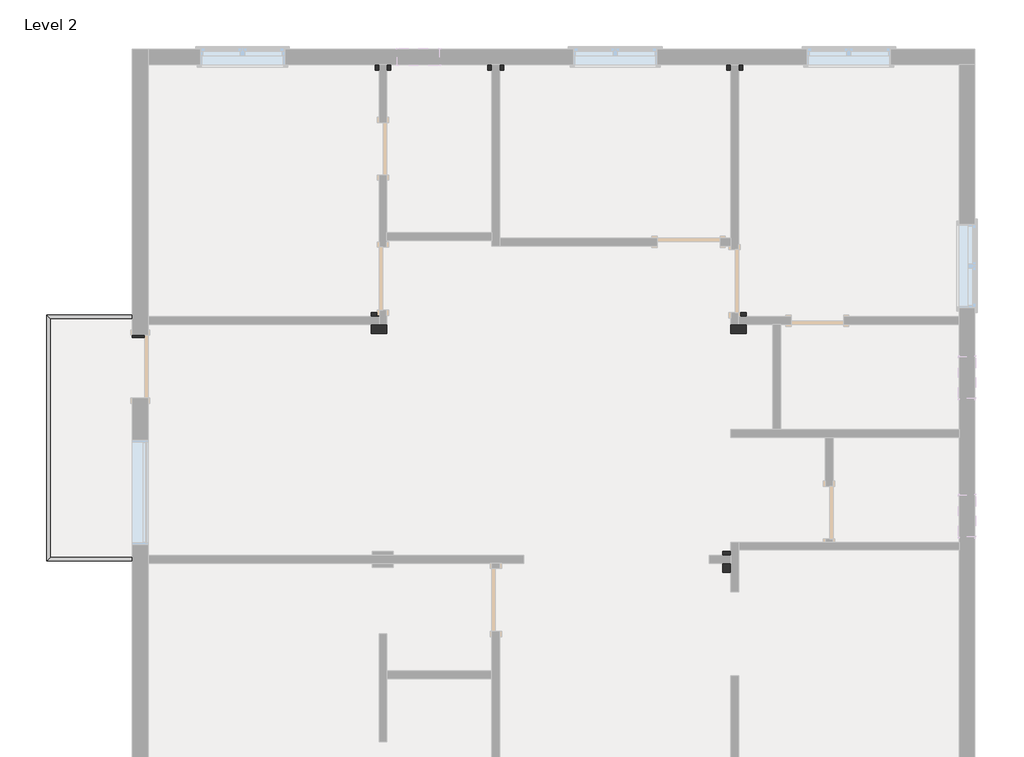
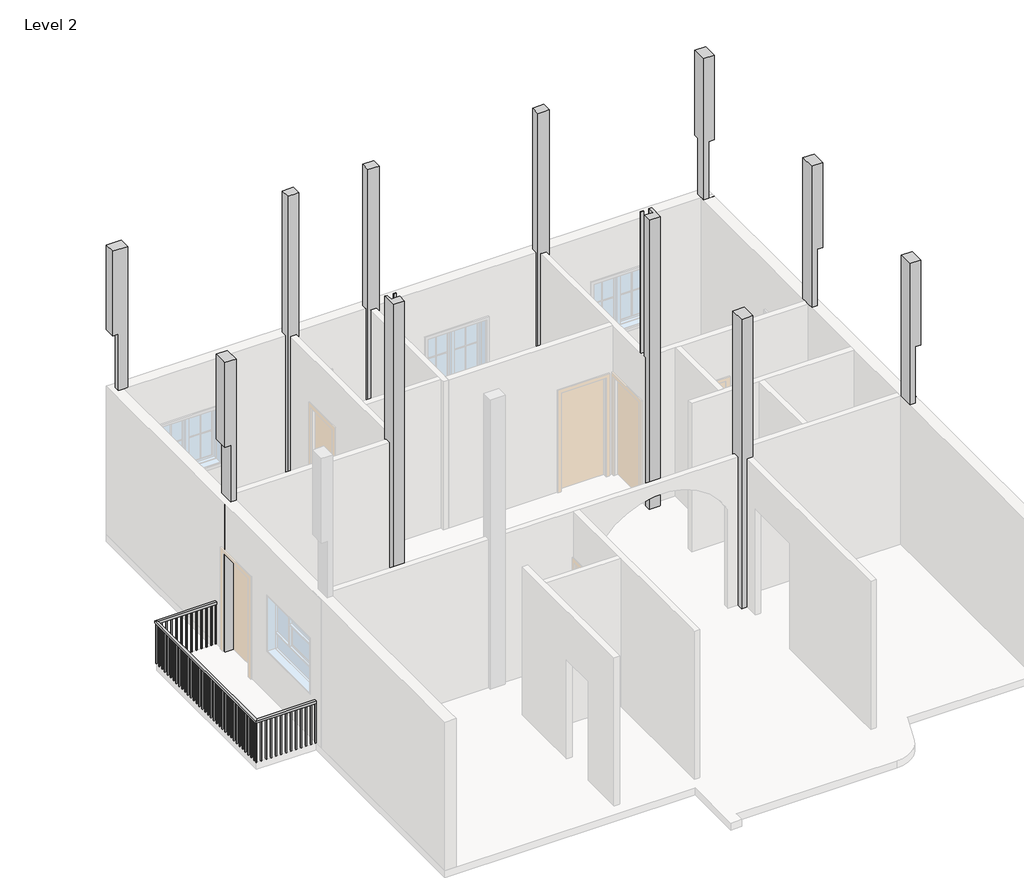
# One storey, part 3 of 4: 11 columns, 1 railing.
"""IFC4 building model written with IfcOpenShell, lengths in millimetres."""

from ifc_helpers import new_model, si_unit, frame, origin, place, context, project, spatial, polyline, outline, extrude, faceted_brep, element, save

model = new_model("IFC4")

# Units and contexts
model_context = context("Model", 3, world=origin())
ifc_project = project(units=[si_unit("LENGTHUNIT", "METRE", prefix="MILLI")], contexts=[model_context])

# Site, building, storey
site = spatial("IfcSite", under=ifc_project)
building = spatial("IfcBuilding", under=site)
storey = spatial("IfcBuildingStorey", under=building, Name="Level 2", Elevation=3200.4)

# Columns
placement = place(None, origin())
element("IfcColumn", 1, ObjectType="Rectangular Column : 9\" x 12\"", at=placement, inside=storey, context=model_context, shape_type="Brep", body=[
    faceted_brep([(-14591.1678125, 13531.616018, 3200.4), (-14591.1678125, 13303.016018, 3200.4), (-14667.3678125, 13303.016018, 3200.4), (-14667.3678125, 13531.616018, 3200.4), (-14591.1678125, 13531.616018, 6400.8), (-14591.1678125, 13417.316018, 6400.8), (-14591.1678125, 13417.316018, 7620.0), (-14591.1678125, 13531.616018, 7620.0), (-14591.1678125, 13531.616018, 9448.8), (-14591.1678125, 13303.016018, 9448.8), (-14895.9678125, 13303.016018, 9448.8), (-14895.9678125, 13303.016018, 7620.0), (-14781.6678125, 13303.016018, 7620.0), (-14781.6678125, 13303.016018, 6400.8), (-14667.3678125, 13303.016018, 6400.8), (-14895.9678125, 13531.616018, 9448.8), (-14895.9678125, 13531.616018, 7620.0), (-14895.9678125, 13417.316018, 7620.0), (-14667.3678125, 13417.316018, 6400.8), (-14667.3678125, 13531.616018, 6400.8), (-14781.6678125, 13417.316018, 6400.8), (-14781.6678125, 13417.316018, 7620.0)], [[[0, 1, 2, 3]], [[1, 0, 4, 5, 6, 7, 8, 9]], [[1, 9, 10, 11, 12, 13, 14, 2]], [[10, 15, 16, 17, 11]], [[15, 8, 7, 16]], [[9, 8, 15, 10]], [[3, 2, 14, 18, 19]], [[14, 13, 20, 18]], [[12, 21, 20, 13]], [[21, 12, 11, 17]], [[5, 18, 20, 21, 6]], [[18, 5, 4, 19]], [[6, 21, 17, 16, 7]], [[0, 3, 19, 4]]]),
])
element("IfcColumn", 2, ObjectType="Rectangular Column : 9\" x 12\"", at=placement, inside=storey, context=model_context, shape_type="Brep", body=[
    faceted_brep([(-11371.7178125, 13226.816018, 3200.4), (-11371.7178125, 13303.016018, 3200.4), (-11314.5678125, 13303.016018, 3200.4), (-11314.5678125, 13226.816018, 3200.4), (-11143.1178125, 13226.816018, 9448.8), (-11143.1178125, 13226.816018, 3200.4), (-11143.1178125, 13303.016018, 3200.4), (-11143.1178125, 13303.016018, 6400.8), (-11143.1178125, 13417.316018, 6400.8), (-11143.1178125, 13417.316018, 9448.8), (-11257.4178125, 13226.816018, 9448.8), (-11371.7178125, 13226.816018, 9448.8), (-11371.7178125, 13226.816018, 6400.8), (-11314.5678125, 13226.816018, 6400.8), (-11257.4178125, 13226.816018, 6400.8), (-11200.2678125, 13226.816018, 6400.8), (-11200.2678125, 13226.816018, 3200.4), (-11371.7178125, 13417.316018, 9448.8), (-11371.7178125, 13417.316018, 6400.8), (-11371.7178125, 13303.016018, 6400.8), (-11314.5678125, 13303.016018, 6400.8), (-11200.2678125, 13303.016018, 6400.8), (-11200.2678125, 13303.016018, 3200.4)], [[[0, 1, 2, 3]], [[4, 5, 6, 7, 8, 9]], [[5, 4, 10, 11, 12, 0, 3, 13, 14, 15, 16]], [[0, 12, 11, 17, 18, 19, 1]], [[11, 10, 4, 9, 17]], [[1, 19, 20, 2]], [[20, 19, 18, 8, 7, 21]], [[20, 13, 3, 2]], [[15, 21, 22, 16]], [[13, 20, 21, 15, 14]], [[6, 5, 16, 22]], [[7, 6, 22, 21]], [[9, 8, 18, 17]]]),
])
element("IfcColumn", 3, ObjectType="Rectangular Column : 9\" x 12\"", at=placement, inside=storey, context=model_context, shape_type="Brep", body=[
    faceted_brep([(-9733.4178125, 13226.816018, 3200.4), (-9733.4178125, 13303.016018, 3200.4), (-9676.2678125, 13303.016018, 3200.4), (-9676.2678125, 13226.816018, 3200.4), (-9504.8178125, 13226.816018, 9448.8), (-9504.8178125, 13226.816018, 3200.4), (-9504.8178125, 13303.016018, 3200.4), (-9504.8178125, 13303.016018, 6400.8), (-9504.8178125, 13417.316018, 6400.8), (-9504.8178125, 13417.316018, 9448.8), (-9733.4178125, 13226.816018, 9448.8), (-9676.2678125, 13226.816018, 6400.8), (-9561.9678125, 13226.816018, 6400.8), (-9561.9678125, 13226.816018, 3200.4), (-9733.4178125, 13417.316018, 9448.8), (-9733.4178125, 13417.316018, 6400.8), (-9733.4178125, 13303.016018, 6400.8), (-9676.2678125, 13303.016018, 6400.8), (-9561.9678125, 13303.016018, 6400.8), (-9561.9678125, 13303.016018, 3200.4)], [[[0, 1, 2, 3]], [[4, 5, 6, 7, 8, 9]], [[5, 4, 10, 0, 3, 11, 12, 13]], [[0, 10, 14, 15, 16, 1]], [[10, 4, 9, 14]], [[1, 16, 17, 2]], [[17, 16, 15, 8, 7, 18]], [[17, 11, 3, 2]], [[12, 18, 19, 13]], [[11, 17, 18, 12]], [[6, 5, 13, 19]], [[7, 6, 19, 18]], [[9, 8, 15, 14]]]),
])
element("IfcColumn", 4, ObjectType="Rectangular Column : 9\" x 12\"", at=placement, inside=storey, context=model_context, shape_type="Brep", body=[
    faceted_brep([(-6266.3178125, 13226.816018, 3200.4), (-6266.3178125, 13303.016018, 3200.4), (-6209.1678125, 13303.016018, 3200.4), (-6209.1678125, 13226.816018, 3200.4), (-6037.7178125, 13226.816018, 9448.8), (-6037.7178125, 13226.816018, 6400.8), (-6037.7178125, 13226.816018, 3200.4), (-6037.7178125, 13303.016018, 3200.4), (-6037.7178125, 13303.016018, 6400.8), (-6037.7178125, 13417.316018, 6400.8), (-6037.7178125, 13417.316018, 9448.8), (-6152.0178125, 13226.816018, 9448.8), (-6266.3178125, 13226.816018, 9448.8), (-6209.1678125, 13226.816018, 6400.8), (-6152.0178125, 13226.816018, 6400.8), (-6094.8678125, 13226.816018, 6400.8), (-6094.8678125, 13226.816018, 3200.4), (-6266.3178125, 13417.316018, 9448.8), (-6266.3178125, 13417.316018, 6400.8), (-6266.3178125, 13303.016018, 6400.8), (-6209.1678125, 13303.016018, 6400.8), (-6094.8678125, 13303.016018, 6400.8), (-6094.8678125, 13303.016018, 3200.4)], [[[0, 1, 2, 3]], [[4, 5, 6, 7, 8, 9, 10]], [[6, 5, 4, 11, 12, 0, 3, 13, 14, 15, 16]], [[0, 12, 17, 18, 19, 1]], [[12, 11, 4, 10, 17]], [[1, 19, 20, 2]], [[20, 19, 18, 9, 8, 21]], [[20, 13, 3, 2]], [[15, 21, 22, 16]], [[13, 20, 21, 15, 14]], [[7, 6, 16, 22]], [[8, 7, 22, 21]], [[10, 9, 18, 17]]]),
])
element("IfcColumn", 5, ObjectType="Rectangular Column : 9\" x 12\"", at=placement, inside=storey, context=model_context, shape_type="Brep", body=[
    faceted_brep([(-2665.8678125, 13226.816018, 3200.4), (-2894.4678125, 13226.816018, 3200.4), (-2894.4678125, 13303.016018, 3200.4), (-2665.8678125, 13303.016018, 3200.4), (-2894.4678125, 13531.616018, 9448.8), (-2665.8678125, 13531.616018, 9448.8), (-2665.8678125, 13531.616018, 7620.0), (-2894.4678125, 13531.616018, 7620.0), (-2665.8678125, 13226.816018, 9448.8), (-2665.8678125, 13226.816018, 7620.0), (-2665.8678125, 13417.316018, 7620.0), (-2665.8678125, 13226.816018, 6400.8), (-2780.1678125, 13226.816018, 6400.8), (-2780.1678125, 13226.816018, 7620.0), (-2894.4678125, 13226.816018, 9448.8), (-2894.4678125, 13417.316018, 7620.0), (-2894.4678125, 13417.316018, 6400.8), (-2894.4678125, 13303.016018, 6400.8), (-2780.1678125, 13303.016018, 6400.8), (-2665.8678125, 13303.016018, 6400.8), (-2780.1678125, 13417.316018, 6400.8), (-2780.1678125, 13417.316018, 7620.0)], [[[0, 1, 2, 3]], [[4, 5, 6, 7]], [[5, 8, 9, 10, 6]], [[1, 0, 11, 12, 13, 9, 8, 14]], [[1, 14, 4, 7, 15, 16, 17, 2]], [[5, 4, 14, 8]], [[3, 2, 17, 18, 19]], [[17, 16, 20, 18]], [[16, 15, 21, 20]], [[7, 6, 10, 21, 15]], [[12, 18, 20, 21, 13]], [[18, 12, 11, 19]], [[13, 21, 10, 9]], [[0, 3, 19, 11]]]),
])
element("IfcColumn", 6, ObjectType="Rectangular Column : 9\" x 12\"", at=placement, inside=storey, context=model_context, shape_type="Brep", body=[
    faceted_brep([(-14895.9678125, 9645.416018, 3200.4), (-14667.3678125, 9645.416018, 3200.4), (-14667.3678125, 9531.116018, 3200.4), (-14667.3678125, 9340.616018, 3200.4), (-14895.9678125, 9340.616018, 3200.4), (-14895.9678125, 9645.416018, 6400.8), (-14781.6678125, 9645.416018, 6400.8), (-14781.6678125, 9645.416018, 7620.0), (-14895.9678125, 9645.416018, 7620.0), (-14895.9678125, 9645.416018, 9448.8), (-14667.3678125, 9645.416018, 9448.8), (-14667.3678125, 9645.416018, 6400.8), (-14667.3678125, 9340.616018, 9448.8), (-14895.9678125, 9340.616018, 9448.8), (-14895.9678125, 9340.616018, 7620.0), (-14781.6678125, 9340.616018, 7620.0), (-14781.6678125, 9340.616018, 6400.8), (-14895.9678125, 9340.616018, 6400.8)], [[[0, 1, 2, 3, 4]], [[1, 0, 5, 6, 7, 8, 9, 10, 11]], [[3, 2, 1, 11, 10, 12]], [[4, 3, 12, 13, 14, 15, 16, 17]], [[13, 9, 8, 14]], [[10, 9, 13, 12]], [[6, 16, 15, 7]], [[16, 6, 5, 17]], [[7, 15, 14, 8]], [[0, 4, 17, 5]]]),
])
element("IfcColumn", 7, ObjectType="Rectangular Column : 9\" x 12\"", at=placement, inside=storey, context=model_context, shape_type="Brep", body=[
    faceted_brep([(-11200.2678125, 9397.766018, 3200.4), (-11428.8678125, 9397.766018, 3200.4), (-11428.8678125, 9531.116018, 3200.4), (-11314.5678125, 9531.116018, 3200.4), (-11200.2678125, 9531.116018, 3200.4), (-11200.2678125, 9397.766018, 9448.8), (-11200.2678125, 9531.116018, 6400.8), (-11200.2678125, 9569.216018, 6400.8), (-11200.2678125, 9569.216018, 9448.8), (-11428.8678125, 9397.766018, 9448.8), (-11428.8678125, 9702.566018, 9448.8), (-11428.8678125, 9702.566018, 3200.4), (-11428.8678125, 9645.416018, 3200.4), (-11428.8678125, 9645.416018, 6400.8), (-11428.8678125, 9531.116018, 6400.8), (-11314.5678125, 9702.566018, 3200.4), (-11314.5678125, 9702.566018, 6400.8), (-11314.5678125, 9645.416018, 6400.8), (-11314.5678125, 9645.416018, 3200.4), (-11314.5678125, 9531.116018, 6400.8), (-11314.5678125, 9569.216018, 6400.8), (-11257.4178125, 9569.216018, 6400.8), (-11371.7178125, 9645.416018, 6400.8), (-11371.7178125, 9569.216018, 6400.8), (-11371.7178125, 9702.566018, 6400.8), (-11371.7178125, 9702.566018, 9448.8), (-11371.7178125, 9569.216018, 9448.8), (-11257.4178125, 9569.216018, 9448.8)], [[[0, 1, 2, 3, 4]], [[5, 0, 4, 6, 7, 8]], [[1, 0, 5, 9]], [[10, 11, 12, 13, 14, 2, 1, 9]], [[15, 16, 17, 18]], [[6, 19, 20, 21, 7]], [[19, 6, 4, 3]], [[14, 19, 3, 2]], [[12, 18, 17, 22, 13]], [[19, 14, 13, 22, 23, 20]], [[11, 15, 18, 12]], [[22, 24, 25, 26, 23]], [[24, 22, 17, 16]], [[23, 26, 27, 21, 20]], [[8, 7, 21, 27]], [[11, 10, 25, 24, 16, 15]], [[9, 5, 8, 27, 26, 25, 10]]]),
    faceted_brep([(-11200.2678125, 9702.566018, 9448.8), (-11200.2678125, 9702.566018, 6400.8), (-11257.4178125, 9702.566018, 6400.8), (-11257.4178125, 9702.566018, 9448.8), (-11257.4178125, 9683.516018, 9448.8), (-11200.2678125, 9683.516018, 9448.8), (-11257.4178125, 9683.516018, 6400.8), (-11200.2678125, 9683.516018, 6400.8)], [[[0, 1, 2, 3]], [[0, 3, 4, 5]], [[3, 2, 6, 4]], [[7, 5, 4, 6]], [[2, 1, 7, 6]], [[1, 0, 5, 7]]]),
])
element("IfcColumn", 8, ObjectType="Rectangular Column : 9\" x 12\"", at=placement, inside=storey, context=model_context, shape_type="Brep", body=[
    faceted_brep([(-5980.5678125, 9397.766018, 3200.4), (-6209.1678125, 9397.766018, 3200.4), (-6209.1678125, 9531.116018, 3200.4), (-6094.8678125, 9531.116018, 3200.4), (-5980.5678125, 9531.116018, 3200.4), (-5980.5678125, 9702.566018, 9448.8), (-5980.5678125, 9702.566018, 3200.4), (-6094.8678125, 9702.566018, 3200.4), (-6094.8678125, 9702.566018, 5334.0), (-6094.8678125, 9702.566018, 6400.8), (-6037.7178125, 9702.566018, 6400.8), (-6037.7178125, 9702.566018, 9448.8), (-5980.5678125, 9397.766018, 9448.8), (-5980.5678125, 9531.116018, 6400.8), (-5980.5678125, 9645.416018, 6400.8), (-5980.5678125, 9645.416018, 3200.4), (-6209.1678125, 9397.766018, 9448.8), (-6209.1678125, 9569.216018, 9448.8), (-6209.1678125, 9569.216018, 6400.8), (-6209.1678125, 9531.116018, 6400.8), (-6094.8678125, 9645.416018, 3200.4), (-6094.8678125, 9645.416018, 6400.8), (-6094.8678125, 9683.516018, 6400.8), (-6094.8678125, 9531.116018, 6400.8), (-6094.8678125, 9569.216018, 6400.8), (-6037.7178125, 9645.416018, 6400.8), (-6037.7178125, 9569.216018, 6400.8), (-6037.7178125, 9569.216018, 9448.8), (-6037.7178125, 9683.516018, 6400.8), (-6037.7178125, 9683.516018, 9448.8)], [[[0, 1, 2, 3, 4]], [[5, 6, 7, 8, 9, 10, 11]], [[6, 5, 12, 0, 4, 13, 14, 15]], [[1, 0, 12, 16]], [[1, 16, 17, 18, 19, 2]], [[8, 7, 20, 21, 22, 9]], [[23, 19, 18, 24]], [[19, 23, 3, 2]], [[23, 13, 4, 3]], [[20, 15, 14, 25, 21]], [[13, 23, 24, 26, 25, 14]], [[7, 6, 15, 20]], [[18, 17, 27, 26, 24]], [[22, 21, 25, 28]], [[26, 27, 29, 28, 25]], [[10, 28, 29, 11]], [[28, 10, 9, 22]], [[12, 5, 11, 29, 27, 17, 16]]]),
    faceted_brep([(-6209.1678125, 9702.566018, 9448.8), (-6209.1678125, 9683.516018, 9448.8), (-6152.0178125, 9683.516018, 9448.8), (-6152.0178125, 9702.566018, 9448.8), (-6209.1678125, 9683.516018, 6400.8), (-6152.0178125, 9683.516018, 6400.8), (-6209.1678125, 9702.566018, 6400.8), (-6152.0178125, 9702.566018, 6400.8)], [[[0, 1, 2, 3]], [[1, 4, 5, 2]], [[4, 6, 7, 5]], [[7, 3, 2, 5]], [[0, 6, 4, 1]], [[6, 0, 3, 7]]]),
])
element("IfcColumn", 9, ObjectType="Rectangular Column : 9\" x 12\"", at=placement, inside=storey, context=model_context, shape_type="Brep", body=[
    faceted_brep([(-2894.4678125, 9702.566018, 3200.4), (-2665.8678125, 9702.566018, 3200.4), (-2665.8678125, 9397.766018, 3200.4), (-2894.4678125, 9397.766018, 3200.4), (-2894.4678125, 9531.116018, 3200.4), (-2894.4678125, 9645.416018, 3200.4), (-2894.4678125, 9702.566018, 9448.8), (-2665.8678125, 9702.566018, 9448.8), (-2665.8678125, 9702.566018, 7620.0), (-2780.1678125, 9702.566018, 7620.0), (-2780.1678125, 9702.566018, 6400.8), (-2665.8678125, 9702.566018, 6400.8), (-2665.8678125, 9397.766018, 9448.8), (-2665.8678125, 9397.766018, 7620.0), (-2665.8678125, 9397.766018, 6400.8), (-2780.1678125, 9397.766018, 6400.8), (-2780.1678125, 9397.766018, 7620.0), (-2894.4678125, 9397.766018, 9448.8)], [[[0, 1, 2, 3, 4, 5]], [[1, 0, 6, 7, 8, 9, 10, 11]], [[7, 12, 13, 8]], [[3, 2, 14, 15, 16, 13, 12, 17]], [[0, 5, 4, 3, 17, 6]], [[7, 6, 17, 12]], [[15, 10, 9, 16]], [[10, 15, 14, 11]], [[16, 9, 8, 13]], [[2, 1, 11, 14]]]),
])
element("IfcColumn", 10, ObjectType="Rectangular Column : 9\" x 12\"", at=placement, inside=storey, context=model_context, shape_type="Brep", body=[
    faceted_brep([(-6323.4678125, 5930.666018, 3200.4), (-6323.4678125, 6064.016018, 3200.4), (-6209.1678125, 6064.016018, 3200.4), (-6209.1678125, 5930.666018, 3200.4), (-6323.4678125, 6235.466018, 9448.8), (-6094.8678125, 6235.466018, 9448.8), (-6094.8678125, 6235.466018, 6400.8), (-6209.1678125, 6235.466018, 6400.8), (-6209.1678125, 6235.466018, 3200.4), (-6323.4678125, 6235.466018, 3200.4), (-6094.8678125, 5930.666018, 9448.8), (-6094.8678125, 5930.666018, 6400.8), (-6323.4678125, 5930.666018, 9448.8), (-6209.1678125, 5930.666018, 6400.8), (-6323.4678125, 6178.316018, 3200.4), (-6323.4678125, 6178.316018, 6400.8), (-6323.4678125, 6064.016018, 6400.8), (-6209.1678125, 6064.016018, 6400.8), (-6209.1678125, 6178.316018, 6400.8), (-6209.1678125, 6178.316018, 3200.4)], [[[0, 1, 2, 3]], [[4, 5, 6, 7, 8, 9]], [[5, 10, 11, 6]], [[10, 12, 0, 3, 13, 11]], [[4, 9, 14, 15, 16, 1, 0, 12]], [[5, 4, 12, 10]], [[16, 17, 2, 1]], [[18, 15, 14, 19]], [[17, 16, 15, 18]], [[7, 18, 19, 8]], [[18, 7, 6, 11, 13, 17]], [[19, 14, 9, 8]], [[17, 13, 3, 2]]]),
])
element("IfcColumn", 11, ObjectType="Rectangular Column : 9\" x 12\"", at=placement, inside=storey, context=model_context, shape_type="SweptSolid", body=[
    extrude(outline(polyline([(3200.4, -2894.4678125), (3200.4, -2665.8678125), (6400.8, -2665.8678125), (6400.8, -2780.1678125), (7620.0, -2780.1678125), (7620.0, -2665.8678125), (9448.8, -2665.8678125), (9448.8, -2894.4678125), (3200.4, -2894.4678125)])), frame((0.0, 5930.666018, 0.0), z_axis=(0.0, 1.0, 0.0), x_axis=(0.0, 0.0, 1.0)), (0.0, 0.0, 1.0), 304.8),
])

# Railing
element("IfcRailing", 12, ObjectType="Handrail - Rectangular", at=placement, inside=storey, context=model_context, shape_type="SolidModel", body=[
    faceted_brep([(-14895.9678125, 9620.016018, 4114.8), (-14895.9678125, 9620.016018, 4064.0), (-14895.9678125, 9670.816018, 4064.0), (-14895.9678125, 9670.816018, 4114.8), (-16089.7678125, 9620.016018, 4114.8), (-16089.7678125, 9620.016018, 4064.0), (-16140.5678125, 9670.816018, 4064.0), (-16140.5678125, 9670.816018, 4114.8), (-16089.7678125, 6146.566018, 4114.8), (-16089.7678125, 6146.566018, 4064.0), (-16140.5678125, 6095.766018, 4064.0), (-16140.5678125, 6095.766018, 4114.8), (-14895.9678125, 6146.566018, 4114.8), (-14895.9678125, 6095.766018, 4114.8), (-14895.9678125, 6095.766018, 4064.0), (-14895.9678125, 6146.566018, 4064.0)], [[[0, 1, 2, 3]], [[1, 0, 4, 5]], [[2, 1, 5, 6]], [[3, 2, 6, 7]], [[0, 3, 7, 4]], [[5, 4, 8, 9]], [[6, 5, 9, 10]], [[7, 6, 10, 11]], [[4, 7, 11, 8]], [[12, 13, 14, 15]], [[9, 8, 12, 15]], [[10, 9, 15, 14]], [[11, 10, 14, 13]], [[8, 11, 13, 12]]]),
    extrude(outline(polyline([(-15007.0928125, 6111.641018), (-15007.0928125, 6130.691018), (-14988.0428125, 6130.691018), (-14988.0428125, 6111.641018), (-15007.0928125, 6111.641018)])), frame((0.0, 0.0, 3200.4), z_axis=(0.0, 0.0, 1.0), x_axis=(1.0, 0.0, 0.0)), (0.0, 0.0, 1.0), 863.6),
    extrude(outline(polyline([(-15108.6928125, 6111.641018), (-15108.6928125, 6130.691018), (-15089.6428125, 6130.691018), (-15089.6428125, 6111.641018), (-15108.6928125, 6111.641018)])), frame((0.0, 0.0, 3200.4), z_axis=(0.0, 0.0, 1.0), x_axis=(1.0, 0.0, 0.0)), (0.0, 0.0, 1.0), 863.6),
    extrude(outline(polyline([(-15210.2928125, 6111.641018), (-15210.2928125, 6130.691018), (-15191.2428125, 6130.691018), (-15191.2428125, 6111.641018), (-15210.2928125, 6111.641018)])), frame((0.0, 0.0, 3200.4), z_axis=(0.0, 0.0, 1.0), x_axis=(1.0, 0.0, 0.0)), (0.0, 0.0, 1.0), 863.6),
    extrude(outline(polyline([(-15311.8928125, 6111.641018), (-15311.8928125, 6130.691018), (-15292.8428125, 6130.691018), (-15292.8428125, 6111.641018), (-15311.8928125, 6111.641018)])), frame((0.0, 0.0, 3200.4), z_axis=(0.0, 0.0, 1.0), x_axis=(1.0, 0.0, 0.0)), (0.0, 0.0, 1.0), 863.6),
    extrude(outline(polyline([(-15413.4928125, 6111.641018), (-15413.4928125, 6130.691018), (-15394.4428125, 6130.691018), (-15394.4428125, 6111.641018), (-15413.4928125, 6111.641018)])), frame((0.0, 0.0, 3200.4), z_axis=(0.0, 0.0, 1.0), x_axis=(1.0, 0.0, 0.0)), (0.0, 0.0, 1.0), 863.6),
    extrude(outline(polyline([(-15515.0928125, 6111.641018), (-15515.0928125, 6130.691018), (-15496.0428125, 6130.691018), (-15496.0428125, 6111.641018), (-15515.0928125, 6111.641018)])), frame((0.0, 0.0, 3200.4), z_axis=(0.0, 0.0, 1.0), x_axis=(1.0, 0.0, 0.0)), (0.0, 0.0, 1.0), 863.6),
    extrude(outline(polyline([(-15616.6928125, 6111.641018), (-15616.6928125, 6130.691018), (-15597.6428125, 6130.691018), (-15597.6428125, 6111.641018), (-15616.6928125, 6111.641018)])), frame((0.0, 0.0, 3200.4), z_axis=(0.0, 0.0, 1.0), x_axis=(1.0, 0.0, 0.0)), (0.0, 0.0, 1.0), 863.6),
    extrude(outline(polyline([(-15718.2928125, 6111.641018), (-15718.2928125, 6130.691018), (-15699.2428125, 6130.691018), (-15699.2428125, 6111.641018), (-15718.2928125, 6111.641018)])), frame((0.0, 0.0, 3200.4), z_axis=(0.0, 0.0, 1.0), x_axis=(1.0, 0.0, 0.0)), (0.0, 0.0, 1.0), 863.6),
    extrude(outline(polyline([(-15819.8928125, 6111.641018), (-15819.8928125, 6130.691018), (-15800.8428125, 6130.691018), (-15800.8428125, 6111.641018), (-15819.8928125, 6111.641018)])), frame((0.0, 0.0, 3200.4), z_axis=(0.0, 0.0, 1.0), x_axis=(1.0, 0.0, 0.0)), (0.0, 0.0, 1.0), 863.6),
    extrude(outline(polyline([(-15921.4928125, 6111.641018), (-15921.4928125, 6130.691018), (-15902.4428125, 6130.691018), (-15902.4428125, 6111.641018), (-15921.4928125, 6111.641018)])), frame((0.0, 0.0, 3200.4), z_axis=(0.0, 0.0, 1.0), x_axis=(1.0, 0.0, 0.0)), (0.0, 0.0, 1.0), 863.6),
    extrude(outline(polyline([(-16023.0928125, 6111.641018), (-16023.0928125, 6130.691018), (-16004.0428125, 6130.691018), (-16004.0428125, 6111.641018), (-16023.0928125, 6111.641018)])), frame((0.0, 0.0, 3200.4), z_axis=(0.0, 0.0, 1.0), x_axis=(1.0, 0.0, 0.0)), (0.0, 0.0, 1.0), 863.6),
    extrude(outline(polyline([(-16124.6928125, 6200.541018), (-16105.6428125, 6200.541018), (-16105.6428125, 6181.491018), (-16124.6928125, 6181.491018), (-16124.6928125, 6200.541018)])), frame((0.0, 0.0, 3200.4), z_axis=(0.0, 0.0, 1.0), x_axis=(1.0, 0.0, 0.0)), (0.0, 0.0, 1.0), 863.6),
    extrude(outline(polyline([(-16124.6928125, 6302.141018), (-16105.6428125, 6302.141018), (-16105.6428125, 6283.091018), (-16124.6928125, 6283.091018), (-16124.6928125, 6302.141018)])), frame((0.0, 0.0, 3200.4), z_axis=(0.0, 0.0, 1.0), x_axis=(1.0, 0.0, 0.0)), (0.0, 0.0, 1.0), 863.6),
    extrude(outline(polyline([(-16124.6928125, 6403.741018), (-16105.6428125, 6403.741018), (-16105.6428125, 6384.691018), (-16124.6928125, 6384.691018), (-16124.6928125, 6403.741018)])), frame((0.0, 0.0, 3200.4), z_axis=(0.0, 0.0, 1.0), x_axis=(1.0, 0.0, 0.0)), (0.0, 0.0, 1.0), 863.6),
    extrude(outline(polyline([(-16124.6928125, 6505.341018), (-16105.6428125, 6505.341018), (-16105.6428125, 6486.291018), (-16124.6928125, 6486.291018), (-16124.6928125, 6505.341018)])), frame((0.0, 0.0, 3200.4), z_axis=(0.0, 0.0, 1.0), x_axis=(1.0, 0.0, 0.0)), (0.0, 0.0, 1.0), 863.6),
    extrude(outline(polyline([(-16124.6928125, 6606.941018), (-16105.6428125, 6606.941018), (-16105.6428125, 6587.891018), (-16124.6928125, 6587.891018), (-16124.6928125, 6606.941018)])), frame((0.0, 0.0, 3200.4), z_axis=(0.0, 0.0, 1.0), x_axis=(1.0, 0.0, 0.0)), (0.0, 0.0, 1.0), 863.6),
    extrude(outline(polyline([(-16124.6928125, 6708.541018), (-16105.6428125, 6708.541018), (-16105.6428125, 6689.491018), (-16124.6928125, 6689.491018), (-16124.6928125, 6708.541018)])), frame((0.0, 0.0, 3200.4), z_axis=(0.0, 0.0, 1.0), x_axis=(1.0, 0.0, 0.0)), (0.0, 0.0, 1.0), 863.6),
    extrude(outline(polyline([(-16124.6928125, 6810.141018), (-16105.6428125, 6810.141018), (-16105.6428125, 6791.091018), (-16124.6928125, 6791.091018), (-16124.6928125, 6810.141018)])), frame((0.0, 0.0, 3200.4), z_axis=(0.0, 0.0, 1.0), x_axis=(1.0, 0.0, 0.0)), (0.0, 0.0, 1.0), 863.6),
    extrude(outline(polyline([(-16124.6928125, 6911.741018), (-16105.6428125, 6911.741018), (-16105.6428125, 6892.691018), (-16124.6928125, 6892.691018), (-16124.6928125, 6911.741018)])), frame((0.0, 0.0, 3200.4), z_axis=(0.0, 0.0, 1.0), x_axis=(1.0, 0.0, 0.0)), (0.0, 0.0, 1.0), 863.6),
    extrude(outline(polyline([(-16124.6928125, 7013.341018), (-16105.6428125, 7013.341018), (-16105.6428125, 6994.291018), (-16124.6928125, 6994.291018), (-16124.6928125, 7013.341018)])), frame((0.0, 0.0, 3200.4), z_axis=(0.0, 0.0, 1.0), x_axis=(1.0, 0.0, 0.0)), (0.0, 0.0, 1.0), 863.6),
    extrude(outline(polyline([(-16124.6928125, 7114.941018), (-16105.6428125, 7114.941018), (-16105.6428125, 7095.891018), (-16124.6928125, 7095.891018), (-16124.6928125, 7114.941018)])), frame((0.0, 0.0, 3200.4), z_axis=(0.0, 0.0, 1.0), x_axis=(1.0, 0.0, 0.0)), (0.0, 0.0, 1.0), 863.6),
    extrude(outline(polyline([(-16124.6928125, 7216.541018), (-16105.6428125, 7216.541018), (-16105.6428125, 7197.491018), (-16124.6928125, 7197.491018), (-16124.6928125, 7216.541018)])), frame((0.0, 0.0, 3200.4), z_axis=(0.0, 0.0, 1.0), x_axis=(1.0, 0.0, 0.0)), (0.0, 0.0, 1.0), 863.6),
    extrude(outline(polyline([(-16124.6928125, 7318.141018), (-16105.6428125, 7318.141018), (-16105.6428125, 7299.091018), (-16124.6928125, 7299.091018), (-16124.6928125, 7318.141018)])), frame((0.0, 0.0, 3200.4), z_axis=(0.0, 0.0, 1.0), x_axis=(1.0, 0.0, 0.0)), (0.0, 0.0, 1.0), 863.6),
    extrude(outline(polyline([(-16124.6928125, 7419.741018), (-16105.6428125, 7419.741018), (-16105.6428125, 7400.691018), (-16124.6928125, 7400.691018), (-16124.6928125, 7419.741018)])), frame((0.0, 0.0, 3200.4), z_axis=(0.0, 0.0, 1.0), x_axis=(1.0, 0.0, 0.0)), (0.0, 0.0, 1.0), 863.6),
    extrude(outline(polyline([(-16124.6928125, 7521.341018), (-16105.6428125, 7521.341018), (-16105.6428125, 7502.291018), (-16124.6928125, 7502.291018), (-16124.6928125, 7521.341018)])), frame((0.0, 0.0, 3200.4), z_axis=(0.0, 0.0, 1.0), x_axis=(1.0, 0.0, 0.0)), (0.0, 0.0, 1.0), 863.6),
    extrude(outline(polyline([(-16124.6928125, 7622.941018), (-16105.6428125, 7622.941018), (-16105.6428125, 7603.891018), (-16124.6928125, 7603.891018), (-16124.6928125, 7622.941018)])), frame((0.0, 0.0, 3200.4), z_axis=(0.0, 0.0, 1.0), x_axis=(1.0, 0.0, 0.0)), (0.0, 0.0, 1.0), 863.6),
    extrude(outline(polyline([(-16124.6928125, 7724.541018), (-16105.6428125, 7724.541018), (-16105.6428125, 7705.491018), (-16124.6928125, 7705.491018), (-16124.6928125, 7724.541018)])), frame((0.0, 0.0, 3200.4), z_axis=(0.0, 0.0, 1.0), x_axis=(1.0, 0.0, 0.0)), (0.0, 0.0, 1.0), 863.6),
    extrude(outline(polyline([(-16124.6928125, 7826.141018), (-16105.6428125, 7826.141018), (-16105.6428125, 7807.091018), (-16124.6928125, 7807.091018), (-16124.6928125, 7826.141018)])), frame((0.0, 0.0, 3200.4), z_axis=(0.0, 0.0, 1.0), x_axis=(1.0, 0.0, 0.0)), (0.0, 0.0, 1.0), 863.6),
    extrude(outline(polyline([(-16124.6928125, 7927.741018), (-16105.6428125, 7927.741018), (-16105.6428125, 7908.691018), (-16124.6928125, 7908.691018), (-16124.6928125, 7927.741018)])), frame((0.0, 0.0, 3200.4), z_axis=(0.0, 0.0, 1.0), x_axis=(1.0, 0.0, 0.0)), (0.0, 0.0, 1.0), 863.6),
    extrude(outline(polyline([(-16124.6928125, 8029.341018), (-16105.6428125, 8029.341018), (-16105.6428125, 8010.291018), (-16124.6928125, 8010.291018), (-16124.6928125, 8029.341018)])), frame((0.0, 0.0, 3200.4), z_axis=(0.0, 0.0, 1.0), x_axis=(1.0, 0.0, 0.0)), (0.0, 0.0, 1.0), 863.6),
    extrude(outline(polyline([(-16124.6928125, 8130.941018), (-16105.6428125, 8130.941018), (-16105.6428125, 8111.891018), (-16124.6928125, 8111.891018), (-16124.6928125, 8130.941018)])), frame((0.0, 0.0, 3200.4), z_axis=(0.0, 0.0, 1.0), x_axis=(1.0, 0.0, 0.0)), (0.0, 0.0, 1.0), 863.6),
    extrude(outline(polyline([(-16124.6928125, 8232.541018), (-16105.6428125, 8232.541018), (-16105.6428125, 8213.491018), (-16124.6928125, 8213.491018), (-16124.6928125, 8232.541018)])), frame((0.0, 0.0, 3200.4), z_axis=(0.0, 0.0, 1.0), x_axis=(1.0, 0.0, 0.0)), (0.0, 0.0, 1.0), 863.6),
    extrude(outline(polyline([(-16124.6928125, 8334.141018), (-16105.6428125, 8334.141018), (-16105.6428125, 8315.091018), (-16124.6928125, 8315.091018), (-16124.6928125, 8334.141018)])), frame((0.0, 0.0, 3200.4), z_axis=(0.0, 0.0, 1.0), x_axis=(1.0, 0.0, 0.0)), (0.0, 0.0, 1.0), 863.6),
    extrude(outline(polyline([(-16124.6928125, 8435.741018), (-16105.6428125, 8435.741018), (-16105.6428125, 8416.691018), (-16124.6928125, 8416.691018), (-16124.6928125, 8435.741018)])), frame((0.0, 0.0, 3200.4), z_axis=(0.0, 0.0, 1.0), x_axis=(1.0, 0.0, 0.0)), (0.0, 0.0, 1.0), 863.6),
    extrude(outline(polyline([(-16124.6928125, 8537.341018), (-16105.6428125, 8537.341018), (-16105.6428125, 8518.291018), (-16124.6928125, 8518.291018), (-16124.6928125, 8537.341018)])), frame((0.0, 0.0, 3200.4), z_axis=(0.0, 0.0, 1.0), x_axis=(1.0, 0.0, 0.0)), (0.0, 0.0, 1.0), 863.6),
    extrude(outline(polyline([(-16124.6928125, 8638.941018), (-16105.6428125, 8638.941018), (-16105.6428125, 8619.891018), (-16124.6928125, 8619.891018), (-16124.6928125, 8638.941018)])), frame((0.0, 0.0, 3200.4), z_axis=(0.0, 0.0, 1.0), x_axis=(1.0, 0.0, 0.0)), (0.0, 0.0, 1.0), 863.6),
    extrude(outline(polyline([(-16124.6928125, 8740.541018), (-16105.6428125, 8740.541018), (-16105.6428125, 8721.491018), (-16124.6928125, 8721.491018), (-16124.6928125, 8740.541018)])), frame((0.0, 0.0, 3200.4), z_axis=(0.0, 0.0, 1.0), x_axis=(1.0, 0.0, 0.0)), (0.0, 0.0, 1.0), 863.6),
    extrude(outline(polyline([(-16124.6928125, 8842.141018), (-16105.6428125, 8842.141018), (-16105.6428125, 8823.091018), (-16124.6928125, 8823.091018), (-16124.6928125, 8842.141018)])), frame((0.0, 0.0, 3200.4), z_axis=(0.0, 0.0, 1.0), x_axis=(1.0, 0.0, 0.0)), (0.0, 0.0, 1.0), 863.6),
    extrude(outline(polyline([(-16124.6928125, 8943.741018), (-16105.6428125, 8943.741018), (-16105.6428125, 8924.691018), (-16124.6928125, 8924.691018), (-16124.6928125, 8943.741018)])), frame((0.0, 0.0, 3200.4), z_axis=(0.0, 0.0, 1.0), x_axis=(1.0, 0.0, 0.0)), (0.0, 0.0, 1.0), 863.6),
    extrude(outline(polyline([(-16124.6928125, 9045.341018), (-16105.6428125, 9045.341018), (-16105.6428125, 9026.291018), (-16124.6928125, 9026.291018), (-16124.6928125, 9045.341018)])), frame((0.0, 0.0, 3200.4), z_axis=(0.0, 0.0, 1.0), x_axis=(1.0, 0.0, 0.0)), (0.0, 0.0, 1.0), 863.6),
    extrude(outline(polyline([(-16124.6928125, 9146.941018), (-16105.6428125, 9146.941018), (-16105.6428125, 9127.891018), (-16124.6928125, 9127.891018), (-16124.6928125, 9146.941018)])), frame((0.0, 0.0, 3200.4), z_axis=(0.0, 0.0, 1.0), x_axis=(1.0, 0.0, 0.0)), (0.0, 0.0, 1.0), 863.6),
    extrude(outline(polyline([(-16124.6928125, 9248.541018), (-16105.6428125, 9248.541018), (-16105.6428125, 9229.491018), (-16124.6928125, 9229.491018), (-16124.6928125, 9248.541018)])), frame((0.0, 0.0, 3200.4), z_axis=(0.0, 0.0, 1.0), x_axis=(1.0, 0.0, 0.0)), (0.0, 0.0, 1.0), 863.6),
    extrude(outline(polyline([(-16124.6928125, 9350.141018), (-16105.6428125, 9350.141018), (-16105.6428125, 9331.091018), (-16124.6928125, 9331.091018), (-16124.6928125, 9350.141018)])), frame((0.0, 0.0, 3200.4), z_axis=(0.0, 0.0, 1.0), x_axis=(1.0, 0.0, 0.0)), (0.0, 0.0, 1.0), 863.6),
    extrude(outline(polyline([(-16124.6928125, 9451.741018), (-16105.6428125, 9451.741018), (-16105.6428125, 9432.691018), (-16124.6928125, 9432.691018), (-16124.6928125, 9451.741018)])), frame((0.0, 0.0, 3200.4), z_axis=(0.0, 0.0, 1.0), x_axis=(1.0, 0.0, 0.0)), (0.0, 0.0, 1.0), 863.6),
    extrude(outline(polyline([(-16124.6928125, 9553.341018), (-16105.6428125, 9553.341018), (-16105.6428125, 9534.291018), (-16124.6928125, 9534.291018), (-16124.6928125, 9553.341018)])), frame((0.0, 0.0, 3200.4), z_axis=(0.0, 0.0, 1.0), x_axis=(1.0, 0.0, 0.0)), (0.0, 0.0, 1.0), 863.6),
    extrude(outline(polyline([(-16004.0428125, 9654.941018), (-16004.0428125, 9635.891018), (-16023.0928125, 9635.891018), (-16023.0928125, 9654.941018), (-16004.0428125, 9654.941018)])), frame((0.0, 0.0, 3200.4), z_axis=(0.0, 0.0, 1.0), x_axis=(1.0, 0.0, 0.0)), (0.0, 0.0, 1.0), 863.6),
    extrude(outline(polyline([(-15902.4428125, 9654.941018), (-15902.4428125, 9635.891018), (-15921.4928125, 9635.891018), (-15921.4928125, 9654.941018), (-15902.4428125, 9654.941018)])), frame((0.0, 0.0, 3200.4), z_axis=(0.0, 0.0, 1.0), x_axis=(1.0, 0.0, 0.0)), (0.0, 0.0, 1.0), 863.6),
    extrude(outline(polyline([(-15800.8428125, 9654.941018), (-15800.8428125, 9635.891018), (-15819.8928125, 9635.891018), (-15819.8928125, 9654.941018), (-15800.8428125, 9654.941018)])), frame((0.0, 0.0, 3200.4), z_axis=(0.0, 0.0, 1.0), x_axis=(1.0, 0.0, 0.0)), (0.0, 0.0, 1.0), 863.6),
    extrude(outline(polyline([(-15699.2428125, 9654.941018), (-15699.2428125, 9635.891018), (-15718.2928125, 9635.891018), (-15718.2928125, 9654.941018), (-15699.2428125, 9654.941018)])), frame((0.0, 0.0, 3200.4), z_axis=(0.0, 0.0, 1.0), x_axis=(1.0, 0.0, 0.0)), (0.0, 0.0, 1.0), 863.6),
    extrude(outline(polyline([(-15597.6428125, 9654.941018), (-15597.6428125, 9635.891018), (-15616.6928125, 9635.891018), (-15616.6928125, 9654.941018), (-15597.6428125, 9654.941018)])), frame((0.0, 0.0, 3200.4), z_axis=(0.0, 0.0, 1.0), x_axis=(1.0, 0.0, 0.0)), (0.0, 0.0, 1.0), 863.6),
    extrude(outline(polyline([(-15496.0428125, 9654.941018), (-15496.0428125, 9635.891018), (-15515.0928125, 9635.891018), (-15515.0928125, 9654.941018), (-15496.0428125, 9654.941018)])), frame((0.0, 0.0, 3200.4), z_axis=(0.0, 0.0, 1.0), x_axis=(1.0, 0.0, 0.0)), (0.0, 0.0, 1.0), 863.6),
    extrude(outline(polyline([(-15394.4428125, 9654.941018), (-15394.4428125, 9635.891018), (-15413.4928125, 9635.891018), (-15413.4928125, 9654.941018), (-15394.4428125, 9654.941018)])), frame((0.0, 0.0, 3200.4), z_axis=(0.0, 0.0, 1.0), x_axis=(1.0, 0.0, 0.0)), (0.0, 0.0, 1.0), 863.6),
    extrude(outline(polyline([(-15292.8428125, 9654.941018), (-15292.8428125, 9635.891018), (-15311.8928125, 9635.891018), (-15311.8928125, 9654.941018), (-15292.8428125, 9654.941018)])), frame((0.0, 0.0, 3200.4), z_axis=(0.0, 0.0, 1.0), x_axis=(1.0, 0.0, 0.0)), (0.0, 0.0, 1.0), 863.6),
    extrude(outline(polyline([(-15191.2428125, 9654.941018), (-15191.2428125, 9635.891018), (-15210.2928125, 9635.891018), (-15210.2928125, 9654.941018), (-15191.2428125, 9654.941018)])), frame((0.0, 0.0, 3200.4), z_axis=(0.0, 0.0, 1.0), x_axis=(1.0, 0.0, 0.0)), (0.0, 0.0, 1.0), 863.6),
    extrude(outline(polyline([(-15089.6428125, 9654.941018), (-15089.6428125, 9635.891018), (-15108.6928125, 9635.891018), (-15108.6928125, 9654.941018), (-15089.6428125, 9654.941018)])), frame((0.0, 0.0, 3200.4), z_axis=(0.0, 0.0, 1.0), x_axis=(1.0, 0.0, 0.0)), (0.0, 0.0, 1.0), 863.6),
    extrude(outline(polyline([(-14988.0428125, 9654.941018), (-14988.0428125, 9635.891018), (-15007.0928125, 9635.891018), (-15007.0928125, 9654.941018), (-14988.0428125, 9654.941018)])), frame((0.0, 0.0, 3200.4), z_axis=(0.0, 0.0, 1.0), x_axis=(1.0, 0.0, 0.0)), (0.0, 0.0, 1.0), 863.6),
    extrude(outline(polyline([(-16124.6928125, 6130.691018), (-16105.6428125, 6130.691018), (-16105.6428125, 6111.641018), (-16124.6928125, 6111.641018), (-16124.6928125, 6130.691018)])), frame((0.0, 0.0, 3200.4), z_axis=(0.0, 0.0, 1.0), x_axis=(1.0, 0.0, 0.0)), (0.0, 0.0, 1.0), 863.6),
    extrude(outline(polyline([(-16105.6428125, 9654.941018), (-16105.6428125, 9635.891018), (-16124.6928125, 9635.891018), (-16124.6928125, 9654.941018), (-16105.6428125, 9654.941018)])), frame((0.0, 0.0, 3200.4), z_axis=(0.0, 0.0, 1.0), x_axis=(1.0, 0.0, 0.0)), (0.0, 0.0, 1.0), 863.6),
    extrude(outline(polyline([(-14915.0178125, 6111.641018), (-14915.0178125, 6130.691018), (-14895.9678125, 6130.691018), (-14895.9678125, 6111.641018), (-14915.0178125, 6111.641018)])), frame((0.0, 0.0, 3200.4), z_axis=(0.0, 0.0, 1.0), x_axis=(1.0, 0.0, 0.0)), (0.0, 0.0, 1.0), 863.6),
    extrude(outline(polyline([(-14895.9678125, 9654.941018), (-14895.9678125, 9635.891018), (-14915.0178125, 9635.891018), (-14915.0178125, 9654.941018), (-14895.9678125, 9654.941018)])), frame((0.0, 0.0, 3200.4), z_axis=(0.0, 0.0, 1.0), x_axis=(1.0, 0.0, 0.0)), (0.0, 0.0, 1.0), 863.6),
])

save(model, "model.ifc")

# Revit data of these elements
# Type "Rectangular Column : 9\" x 12\""
#   Assembly Code = "B1010200"
#   Depth = 0' - 9"
#   Offset Base = 0' - 0"
#   Offset Top = 0' - 0"
#   Width = 1' - 0"
#   Material = none
# Type "Handrail - Rectangular"
#   Assembly Code = "C2010400"
#   built-in parameter 1008612 = 0.0416667 (stored number, unit not read)
#   built-in parameter 1008611 = 0.0416667 (stored number, unit not read)
#   built-in parameter 1008609 = 0.333333 (stored number, unit not read)
#   built-in parameter 1008604 = 0.166667 (stored number, unit not read)
#   built-in parameter 1008603 = 0.166667 (stored number, unit not read)
#   Railing Height = 3' - 0"
#   built-in parameter 1008630 = 2
#   built-in parameter 1008610 = 2
#   built-in parameter 1008618 = Baluster - Square : 3/4"
# Elements 1, 2, 3, 4, 5, 6, 7, 8, 9, 10, 11 (IfcColumn, "Rectangular Column : 9\" x 12\"")
#   Phase Created = New Construction
#   Materials on its faces: "Gypsum Wall Board"
# Element 12 (IfcRailing, "Handrail - Rectangular")
#   Phase Created = New Construction
# Materials
#   "Gypsum Wall Board": class "Generic", colour RGB 127 127 127, transparency 0, Description = "Gypsum Wall Board", Cost = 0
